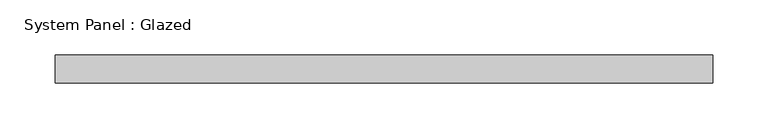
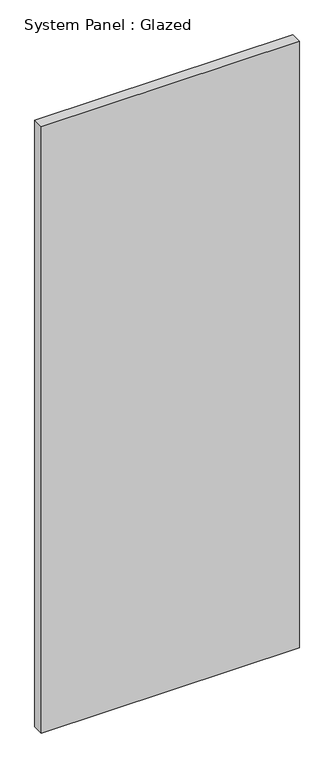
"""IFC4 building model written with IfcOpenShell, lengths in millimetres: plate geometry, System Panel : Glazed."""

from ifc_helpers import new_model, si_unit, origin, origin_with_axes, place, context, project, spatial, polyline, outline, extrude, source, transform, mapped, element, save


def system_panel_glazed_b36345c5(model_context):
    return source(origin(), model_context, "Body", "SweptSolid", [
        extrude(outline(polyline([(298.45, 19.05), (-298.45, 19.05), (-298.45, 44.45), (298.45, 44.45), (298.45, 19.05)])), origin_with_axes(), (0.0, 0.0, 1.0), 1481.6208916),
    ])


if __name__ == "__main__":
    model = new_model("IFC4")
    model_context = context("Model", 3, world=origin())
    ifc_project = project(units=[si_unit("LENGTHUNIT", "METRE", prefix="MILLI")], contexts=[model_context])
    site = spatial("IfcSite", under=ifc_project)
    building = spatial("IfcBuilding", under=site)
    placement = place(None, origin())
    system_panel_glazed_shape = system_panel_glazed_b36345c5(model_context)
    element("IfcPlate", 1, ObjectType="System Panel : Glazed", at=placement, inside=building, context=model_context, shape_type="MappedRepresentation", body=[
        mapped(system_panel_glazed_shape, transform((0.0, 0.0, 0.0), x_axis=(1.0, 0.0, 0.0), y_axis=(0.0, 1.0, 0.0), z_axis=(0.0, 0.0, 1.0))),
    ])
    save(model, "model.ifc")

# Revit data of these elements
# Type "System Panel : Glazed"
#   Construction Type Id = "GSP4R"
#   Analytic Construction = "1/8 in Pilkington single glazing"
#   Visual Light Transmittance = 0.9
#   Solar Heat Gain Coefficient = 0.86
#   Heat Transfer Coefficient (U) = 1.18115 BTU/(h·ft²·°F)
#   Define Thermal Properties by = 1
# Element 1 (IfcPlate, "System Panel : Glazed")
#   Materials on its faces: "Glass"
# Materials
#   "Glass": class "Glass", colour RGB 0 128 192, transparency 0.75, Description = "Soda Lime Glass", Cost = 0
